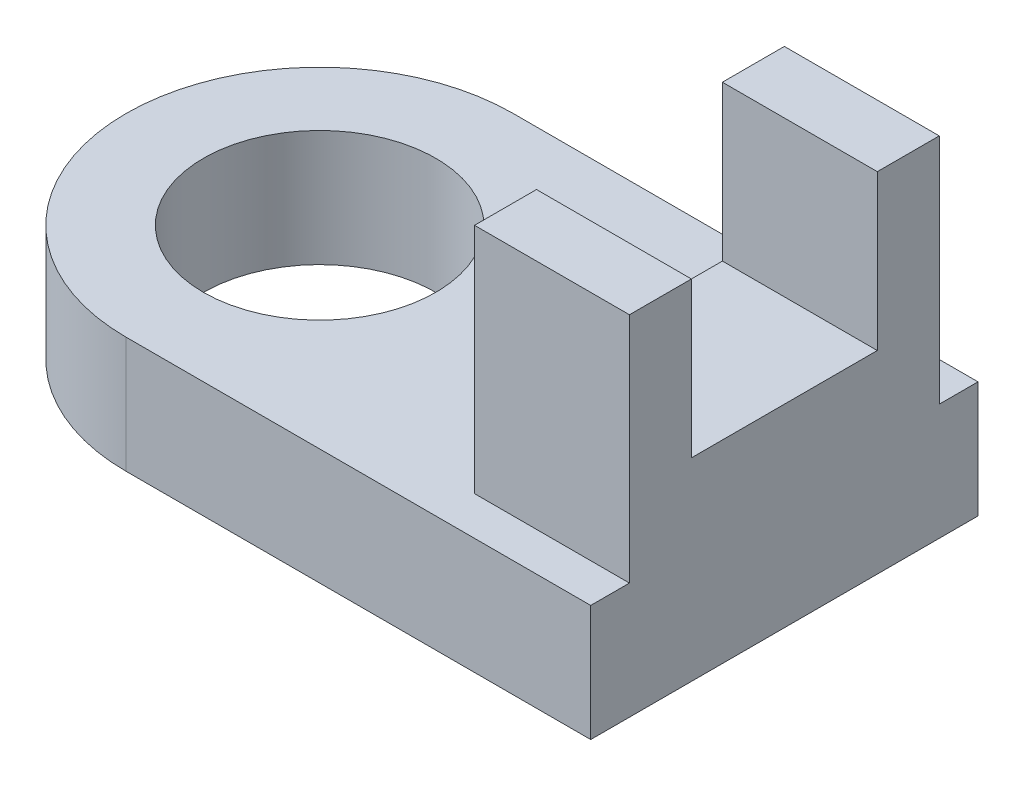
ISO-10303-21;
HEADER;
FILE_DESCRIPTION(('STEP AP214'),'2;1');
FILE_NAME('part.step','',(''),(''),'','','');
FILE_SCHEMA(('AUTOMOTIVE_DESIGN { 1 0 10303 214 1 1 1 1 }'));
ENDSEC;
DATA;
#1=APPLICATION_CONTEXT('core data for automotive mechanical design processes');
#2=APPLICATION_PROTOCOL_DEFINITION('international standard','automotive_design',2000,#1);
#3=PRODUCT_CONTEXT('',#1,'mechanical');
#4=PRODUCT('Part','Part','',(#3));
#5=PRODUCT_RELATED_PRODUCT_CATEGORY('part','',(#4));
#6=PRODUCT_DEFINITION_FORMATION('','',#4);
#7=PRODUCT_DEFINITION_CONTEXT('part definition',#1,'design');
#8=PRODUCT_DEFINITION('design','',#6,#7);
#9=PRODUCT_DEFINITION_SHAPE('','',#8);
#10=(LENGTH_UNIT() NAMED_UNIT(*) SI_UNIT(.MILLI.,.METRE.));
#11=(NAMED_UNIT(*) PLANE_ANGLE_UNIT() SI_UNIT($,.RADIAN.));
#12=(NAMED_UNIT(*) SI_UNIT($,.STERADIAN.) SOLID_ANGLE_UNIT());
#13=UNCERTAINTY_MEASURE_WITH_UNIT(LENGTH_MEASURE(1.E-05),#10,'distance_accuracy_value','');
#14=(GEOMETRIC_REPRESENTATION_CONTEXT(3) GLOBAL_UNCERTAINTY_ASSIGNED_CONTEXT((#13)) GLOBAL_UNIT_ASSIGNED_CONTEXT((#10,
#11,#12)) REPRESENTATION_CONTEXT('',''));
#15=CARTESIAN_POINT('',(0.,0.,0.));
#16=DIRECTION('',(0.,0.,1.));
#17=DIRECTION('',(1.,0.,0.));
#18=AXIS2_PLACEMENT_3D('',#15,#16,#17);
#19=CARTESIAN_POINT('',(-30.,7.5,25.));
#20=DIRECTION('',(0.,-1.,0.));
#21=DIRECTION('',(0.,0.,-1.));
#22=AXIS2_PLACEMENT_3D('',#19,#20,#21);
#23=PLANE('',#22);
#24=CARTESIAN_POINT('',(-30.,7.5,0.));
#25=DIRECTION('',(0.,1.,0.));
#26=DIRECTION('',(0.,0.,1.));
#27=AXIS2_PLACEMENT_3D('',#24,#25,#26);
#28=CIRCLE('',#27,15.);
#29=CARTESIAN_POINT('',(-30.,7.5,15.));
#30=VERTEX_POINT('',#29);
#31=EDGE_CURVE('E160',#30,#30,#28,.T.);
#32=ORIENTED_EDGE('',*,*,#31,.F.);
#33=EDGE_LOOP('',(#32));
#34=FACE_BOUND('',#33,.T.);
#35=DIRECTION('',(1.,0.,0.));
#36=VECTOR('',#35,1.);
#37=CARTESIAN_POINT('',(10.,7.49999999999999,20.));
#38=LINE('',#37,#36);
#39=CARTESIAN_POINT('',(10.,7.49999999999999,20.));
#40=VERTEX_POINT('',#39);
#41=CARTESIAN_POINT('',(30.,7.5,20.));
#42=VERTEX_POINT('',#41);
#43=EDGE_CURVE('E207',#40,#42,#38,.T.);
#44=ORIENTED_EDGE('',*,*,#43,.F.);
#45=DIRECTION('',(0.,0.,-1.));
#46=VECTOR('',#45,1.);
#47=CARTESIAN_POINT('',(10.,7.5,-20.));
#48=LINE('',#47,#46);
#49=CARTESIAN_POINT('',(10.,7.5,-20.));
#50=VERTEX_POINT('',#49);
#51=EDGE_CURVE('E164',#40,#50,#48,.T.);
#52=ORIENTED_EDGE('',*,*,#51,.T.);
#53=DIRECTION('',(1.,0.,0.));
#54=VECTOR('',#53,1.);
#55=CARTESIAN_POINT('',(10.,7.5,-20.));
#56=LINE('',#55,#54);
#57=CARTESIAN_POINT('',(30.,7.5,-20.));
#58=VERTEX_POINT('',#57);
#59=EDGE_CURVE('E187',#50,#58,#56,.T.);
#60=ORIENTED_EDGE('',*,*,#59,.T.);
#61=DIRECTION('',(0.,0.,-1.));
#62=VECTOR('',#61,1.);
#63=CARTESIAN_POINT('',(30.,7.5,25.));
#64=LINE('',#63,#62);
#65=CARTESIAN_POINT('',(30.,7.5,-25.));
#66=VERTEX_POINT('',#65);
#67=EDGE_CURVE('E47',#58,#66,#64,.T.);
#68=ORIENTED_EDGE('',*,*,#67,.T.);
#69=DIRECTION('',(-1.,0.,0.));
#70=VECTOR('',#69,1.);
#71=CARTESIAN_POINT('',(-30.,7.5,-25.));
#72=LINE('',#71,#70);
#73=CARTESIAN_POINT('',(-30.,7.5,-25.));
#74=VERTEX_POINT('',#73);
#75=EDGE_CURVE('E153',#66,#74,#72,.T.);
#76=ORIENTED_EDGE('',*,*,#75,.T.);
#77=CARTESIAN_POINT('',(-30.,7.5,0.));
#78=DIRECTION('',(0.,1.,0.));
#79=DIRECTION('',(0.,0.,1.));
#80=AXIS2_PLACEMENT_3D('',#77,#78,#79);
#81=CIRCLE('',#80,25.);
#82=CARTESIAN_POINT('',(-30.,7.5,25.));
#83=VERTEX_POINT('',#82);
#84=EDGE_CURVE('E155',#74,#83,#81,.T.);
#85=ORIENTED_EDGE('',*,*,#84,.T.);
#86=DIRECTION('',(-1.,0.,0.));
#87=VECTOR('',#86,1.);
#88=CARTESIAN_POINT('',(-30.,7.5,25.));
#89=LINE('',#88,#87);
#90=CARTESIAN_POINT('',(30.,7.5,25.));
#91=VERTEX_POINT('',#90);
#92=EDGE_CURVE('E90',#91,#83,#89,.T.);
#93=ORIENTED_EDGE('',*,*,#92,.F.);
#94=EDGE_CURVE('E11',#91,#42,#64,.T.);
#95=ORIENTED_EDGE('',*,*,#94,.T.);
#96=EDGE_LOOP('',(#44,#52,#60,#68,#76,#85,#93,#95));
#97=FACE_BOUND('',#96,.T.);
#98=ADVANCED_FACE('F41',(#34,#97),#23,.F.);
#99=CARTESIAN_POINT('',(30.,7.5,25.));
#100=DIRECTION('',(-1.,0.,0.));
#101=DIRECTION('',(0.,-1.,0.));
#102=AXIS2_PLACEMENT_3D('',#99,#100,#101);
#103=PLANE('',#102);
#104=DIRECTION('',(0.,1.,0.));
#105=VECTOR('',#104,1.);
#106=CARTESIAN_POINT('',(30.,7.5,-25.));
#107=LINE('',#106,#105);
#108=CARTESIAN_POINT('',(30.,-7.5,-25.));
#109=VERTEX_POINT('',#108);
#110=EDGE_CURVE('E148',#109,#66,#107,.T.);
#111=ORIENTED_EDGE('',*,*,#110,.T.);
#112=ORIENTED_EDGE('',*,*,#67,.F.);
#113=DIRECTION('',(0.,1.,0.));
#114=VECTOR('',#113,1.);
#115=CARTESIAN_POINT('',(30.,37.5,-20.));
#116=LINE('',#115,#114);
#117=CARTESIAN_POINT('',(30.,37.5,-20.));
#118=VERTEX_POINT('',#117);
#119=EDGE_CURVE('E57',#58,#118,#116,.T.);
#120=ORIENTED_EDGE('',*,*,#119,.T.);
#121=DIRECTION('',(0.,0.,1.));
#122=VECTOR('',#121,1.);
#123=CARTESIAN_POINT('',(30.,37.5,-12.));
#124=LINE('',#123,#122);
#125=CARTESIAN_POINT('',(30.,37.5,-12.));
#126=VERTEX_POINT('',#125);
#127=EDGE_CURVE('E195',#118,#126,#124,.T.);
#128=ORIENTED_EDGE('',*,*,#127,.T.);
#129=DIRECTION('',(0.,-1.,0.));
#130=VECTOR('',#129,1.);
#131=CARTESIAN_POINT('',(30.,17.5,-12.));
#132=LINE('',#131,#130);
#133=CARTESIAN_POINT('',(30.,17.5,-12.));
#134=VERTEX_POINT('',#133);
#135=EDGE_CURVE('E192',#126,#134,#132,.T.);
#136=ORIENTED_EDGE('',*,*,#135,.T.);
#137=DIRECTION('',(0.,0.,1.));
#138=VECTOR('',#137,1.);
#139=CARTESIAN_POINT('',(30.,17.5,12.));
#140=LINE('',#139,#138);
#141=CARTESIAN_POINT('',(30.,17.5,12.));
#142=VERTEX_POINT('',#141);
#143=EDGE_CURVE('E196',#134,#142,#140,.T.);
#144=ORIENTED_EDGE('',*,*,#143,.T.);
#145=DIRECTION('',(0.,1.,0.));
#146=VECTOR('',#145,1.);
#147=CARTESIAN_POINT('',(30.,37.5,12.));
#148=LINE('',#147,#146);
#149=CARTESIAN_POINT('',(30.,37.5,12.));
#150=VERTEX_POINT('',#149);
#151=EDGE_CURVE('E203',#142,#150,#148,.T.);
#152=ORIENTED_EDGE('',*,*,#151,.T.);
#153=DIRECTION('',(0.,0.,1.));
#154=VECTOR('',#153,1.);
#155=CARTESIAN_POINT('',(30.,37.5,20.));
#156=LINE('',#155,#154);
#157=CARTESIAN_POINT('',(30.,37.5,20.));
#158=VERTEX_POINT('',#157);
#159=EDGE_CURVE('E204',#150,#158,#156,.T.);
#160=ORIENTED_EDGE('',*,*,#159,.T.);
#161=DIRECTION('',(0.,-1.,0.));
#162=VECTOR('',#161,1.);
#163=CARTESIAN_POINT('',(30.,7.5,20.));
#164=LINE('',#163,#162);
#165=EDGE_CURVE('E166',#158,#42,#164,.T.);
#166=ORIENTED_EDGE('',*,*,#165,.T.);
#167=ORIENTED_EDGE('',*,*,#94,.F.);
#168=DIRECTION('',(0.,1.,0.));
#169=VECTOR('',#168,1.);
#170=CARTESIAN_POINT('',(30.,7.5,25.));
#171=LINE('',#170,#169);
#172=CARTESIAN_POINT('',(30.,-7.5,25.));
#173=VERTEX_POINT('',#172);
#174=EDGE_CURVE('E150',#173,#91,#171,.T.);
#175=ORIENTED_EDGE('',*,*,#174,.F.);
#176=DIRECTION('',(0.,0.,-1.));
#177=VECTOR('',#176,1.);
#178=CARTESIAN_POINT('',(30.,-7.5,25.));
#179=LINE('',#178,#177);
#180=EDGE_CURVE('E228',#173,#109,#179,.T.);
#181=ORIENTED_EDGE('',*,*,#180,.T.);
#182=EDGE_LOOP('',(#111,#112,#120,#128,#136,#144,#152,#160,#166,#167,#175,#181));
#183=FACE_BOUND('',#182,.T.);
#184=ADVANCED_FACE('F43',(#183),#103,.F.);
#185=CARTESIAN_POINT('',(-30.,-7.5,25.));
#186=DIRECTION('',(0.,1.,0.));
#187=DIRECTION('',(0.,0.,1.));
#188=AXIS2_PLACEMENT_3D('',#185,#186,#187);
#189=PLANE('',#188);
#190=CARTESIAN_POINT('',(-30.,-7.5,0.));
#191=DIRECTION('',(0.,1.,0.));
#192=DIRECTION('',(0.,0.,1.));
#193=AXIS2_PLACEMENT_3D('',#190,#191,#192);
#194=CIRCLE('',#193,15.);
#195=CARTESIAN_POINT('',(-30.,-7.5,15.));
#196=VERTEX_POINT('',#195);
#197=EDGE_CURVE('E156',#196,#196,#194,.T.);
#198=ORIENTED_EDGE('',*,*,#197,.T.);
#199=EDGE_LOOP('',(#198));
#200=FACE_BOUND('',#199,.T.);
#201=DIRECTION('',(1.,0.,0.));
#202=VECTOR('',#201,1.);
#203=CARTESIAN_POINT('',(-30.,-7.5,-25.));
#204=LINE('',#203,#202);
#205=CARTESIAN_POINT('',(-30.,-7.5,-25.));
#206=VERTEX_POINT('',#205);
#207=EDGE_CURVE('E81',#206,#109,#204,.T.);
#208=ORIENTED_EDGE('',*,*,#207,.T.);
#209=ORIENTED_EDGE('',*,*,#180,.F.);
#210=DIRECTION('',(1.,0.,0.));
#211=VECTOR('',#210,1.);
#212=CARTESIAN_POINT('',(-30.,-7.5,25.));
#213=LINE('',#212,#211);
#214=CARTESIAN_POINT('',(-30.,-7.5,25.));
#215=VERTEX_POINT('',#214);
#216=EDGE_CURVE('E62',#215,#173,#213,.T.);
#217=ORIENTED_EDGE('',*,*,#216,.F.);
#218=CARTESIAN_POINT('',(-30.,-7.5,0.));
#219=DIRECTION('',(0.,1.,0.));
#220=DIRECTION('',(0.,0.,1.));
#221=AXIS2_PLACEMENT_3D('',#218,#219,#220);
#222=CIRCLE('',#221,25.);
#223=EDGE_CURVE('E151',#206,#215,#222,.T.);
#224=ORIENTED_EDGE('',*,*,#223,.F.);
#225=EDGE_LOOP('',(#208,#209,#217,#224));
#226=FACE_BOUND('',#225,.T.);
#227=ADVANCED_FACE('F154',(#200,#226),#189,.F.);
#228=CARTESIAN_POINT('',(0.,0.,25.));
#229=DIRECTION('',(0.,0.,1.));
#230=DIRECTION('',(1.,0.,0.));
#231=AXIS2_PLACEMENT_3D('',#228,#229,#230);
#232=PLANE('',#231);
#233=ORIENTED_EDGE('',*,*,#174,.T.);
#234=ORIENTED_EDGE('',*,*,#92,.T.);
#235=DIRECTION('',(0.,-1.,0.));
#236=VECTOR('',#235,1.);
#237=CARTESIAN_POINT('',(-30.,7.5,25.));
#238=LINE('',#237,#236);
#239=EDGE_CURVE('E229',#83,#215,#238,.T.);
#240=ORIENTED_EDGE('',*,*,#239,.T.);
#241=ORIENTED_EDGE('',*,*,#216,.T.);
#242=EDGE_LOOP('',(#233,#234,#240,#241));
#243=FACE_BOUND('',#242,.T.);
#244=ADVANCED_FACE('F238',(#243),#232,.T.);
#245=CARTESIAN_POINT('',(0.,0.,-25.));
#246=DIRECTION('',(0.,0.,1.));
#247=DIRECTION('',(1.,0.,0.));
#248=AXIS2_PLACEMENT_3D('',#245,#246,#247);
#249=PLANE('',#248);
#250=ORIENTED_EDGE('',*,*,#110,.F.);
#251=ORIENTED_EDGE('',*,*,#207,.F.);
#252=DIRECTION('',(0.,-1.,0.));
#253=VECTOR('',#252,1.);
#254=CARTESIAN_POINT('',(-30.,7.5,-25.));
#255=LINE('',#254,#253);
#256=EDGE_CURVE('E141',#74,#206,#255,.T.);
#257=ORIENTED_EDGE('',*,*,#256,.F.);
#258=ORIENTED_EDGE('',*,*,#75,.F.);
#259=EDGE_LOOP('',(#250,#251,#257,#258));
#260=FACE_BOUND('',#259,.T.);
#261=ADVANCED_FACE('F143',(#260),#249,.F.);
#262=CARTESIAN_POINT('',(10.,7.49999999999999,20.));
#263=DIRECTION('',(0.,0.,1.));
#264=DIRECTION('',(1.,0.,0.));
#265=AXIS2_PLACEMENT_3D('',#262,#263,#264);
#266=PLANE('',#265);
#267=ORIENTED_EDGE('',*,*,#165,.F.);
#268=DIRECTION('',(1.,0.,0.));
#269=VECTOR('',#268,1.);
#270=CARTESIAN_POINT('',(9.99999999999999,37.5,20.));
#271=LINE('',#270,#269);
#272=CARTESIAN_POINT('',(9.99999999999999,37.5,20.));
#273=VERTEX_POINT('',#272);
#274=EDGE_CURVE('E211',#273,#158,#271,.T.);
#275=ORIENTED_EDGE('',*,*,#274,.F.);
#276=DIRECTION('',(0.,-1.,0.));
#277=VECTOR('',#276,1.);
#278=CARTESIAN_POINT('',(10.,7.49999999999999,20.));
#279=LINE('',#278,#277);
#280=EDGE_CURVE('E186',#273,#40,#279,.T.);
#281=ORIENTED_EDGE('',*,*,#280,.T.);
#282=ORIENTED_EDGE('',*,*,#43,.T.);
#283=EDGE_LOOP('',(#267,#275,#281,#282));
#284=FACE_BOUND('',#283,.T.);
#285=ADVANCED_FACE('F252',(#284),#266,.T.);
#286=CARTESIAN_POINT('',(9.99999999999999,37.5,20.));
#287=DIRECTION('',(0.,1.,0.));
#288=DIRECTION('',(-1.,0.,0.));
#289=AXIS2_PLACEMENT_3D('',#286,#287,#288);
#290=PLANE('',#289);
#291=ORIENTED_EDGE('',*,*,#159,.F.);
#292=DIRECTION('',(1.,0.,0.));
#293=VECTOR('',#292,1.);
#294=CARTESIAN_POINT('',(9.99999999999999,37.5,12.));
#295=LINE('',#294,#293);
#296=CARTESIAN_POINT('',(9.99999999999999,37.5,12.));
#297=VERTEX_POINT('',#296);
#298=EDGE_CURVE('E213',#297,#150,#295,.T.);
#299=ORIENTED_EDGE('',*,*,#298,.F.);
#300=DIRECTION('',(0.,0.,1.));
#301=VECTOR('',#300,1.);
#302=CARTESIAN_POINT('',(9.99999999999999,37.5,20.));
#303=LINE('',#302,#301);
#304=EDGE_CURVE('E184',#297,#273,#303,.T.);
#305=ORIENTED_EDGE('',*,*,#304,.T.);
#306=ORIENTED_EDGE('',*,*,#274,.T.);
#307=EDGE_LOOP('',(#291,#299,#305,#306));
#308=FACE_BOUND('',#307,.T.);
#309=ADVANCED_FACE('F273',(#308),#290,.T.);
#310=CARTESIAN_POINT('',(9.99999999999999,37.5,12.));
#311=DIRECTION('',(0.,0.,-1.));
#312=DIRECTION('',(0.,1.,0.));
#313=AXIS2_PLACEMENT_3D('',#310,#311,#312);
#314=PLANE('',#313);
#315=ORIENTED_EDGE('',*,*,#151,.F.);
#316=DIRECTION('',(1.,0.,0.));
#317=VECTOR('',#316,1.);
#318=CARTESIAN_POINT('',(10.,17.5,12.));
#319=LINE('',#318,#317);
#320=CARTESIAN_POINT('',(10.,17.5,12.));
#321=VERTEX_POINT('',#320);
#322=EDGE_CURVE('E214',#321,#142,#319,.T.);
#323=ORIENTED_EDGE('',*,*,#322,.F.);
#324=DIRECTION('',(0.,1.,0.));
#325=VECTOR('',#324,1.);
#326=CARTESIAN_POINT('',(9.99999999999999,37.5,12.));
#327=LINE('',#326,#325);
#328=EDGE_CURVE('E182',#321,#297,#327,.T.);
#329=ORIENTED_EDGE('',*,*,#328,.T.);
#330=ORIENTED_EDGE('',*,*,#298,.T.);
#331=EDGE_LOOP('',(#315,#323,#329,#330));
#332=FACE_BOUND('',#331,.T.);
#333=ADVANCED_FACE('F269',(#332),#314,.T.);
#334=CARTESIAN_POINT('',(10.,17.5,12.));
#335=DIRECTION('',(0.,1.,0.));
#336=DIRECTION('',(-1.,0.,0.));
#337=AXIS2_PLACEMENT_3D('',#334,#335,#336);
#338=PLANE('',#337);
#339=ORIENTED_EDGE('',*,*,#143,.F.);
#340=DIRECTION('',(1.,0.,0.));
#341=VECTOR('',#340,1.);
#342=CARTESIAN_POINT('',(10.,17.5,-12.));
#343=LINE('',#342,#341);
#344=CARTESIAN_POINT('',(10.,17.5,-12.));
#345=VERTEX_POINT('',#344);
#346=EDGE_CURVE('E220',#345,#134,#343,.T.);
#347=ORIENTED_EDGE('',*,*,#346,.F.);
#348=DIRECTION('',(0.,0.,1.));
#349=VECTOR('',#348,1.);
#350=CARTESIAN_POINT('',(10.,17.5,12.));
#351=LINE('',#350,#349);
#352=EDGE_CURVE('E176',#345,#321,#351,.T.);
#353=ORIENTED_EDGE('',*,*,#352,.T.);
#354=ORIENTED_EDGE('',*,*,#322,.T.);
#355=EDGE_LOOP('',(#339,#347,#353,#354));
#356=FACE_BOUND('',#355,.T.);
#357=ADVANCED_FACE('F266',(#356),#338,.T.);
#358=CARTESIAN_POINT('',(10.,17.5,-12.));
#359=DIRECTION('',(0.,0.,1.));
#360=DIRECTION('',(1.,0.,0.));
#361=AXIS2_PLACEMENT_3D('',#358,#359,#360);
#362=PLANE('',#361);
#363=ORIENTED_EDGE('',*,*,#135,.F.);
#364=DIRECTION('',(1.,0.,0.));
#365=VECTOR('',#364,1.);
#366=CARTESIAN_POINT('',(9.99999999999999,37.5,-12.));
#367=LINE('',#366,#365);
#368=CARTESIAN_POINT('',(9.99999999999999,37.5,-12.));
#369=VERTEX_POINT('',#368);
#370=EDGE_CURVE('E218',#369,#126,#367,.T.);
#371=ORIENTED_EDGE('',*,*,#370,.F.);
#372=DIRECTION('',(0.,-1.,0.));
#373=VECTOR('',#372,1.);
#374=CARTESIAN_POINT('',(10.,17.5,-12.));
#375=LINE('',#374,#373);
#376=EDGE_CURVE('E172',#369,#345,#375,.T.);
#377=ORIENTED_EDGE('',*,*,#376,.T.);
#378=ORIENTED_EDGE('',*,*,#346,.T.);
#379=EDGE_LOOP('',(#363,#371,#377,#378));
#380=FACE_BOUND('',#379,.T.);
#381=ADVANCED_FACE('F265',(#380),#362,.T.);
#382=CARTESIAN_POINT('',(9.99999999999999,37.5,-12.));
#383=DIRECTION('',(0.,1.,0.));
#384=DIRECTION('',(-1.,0.,0.));
#385=AXIS2_PLACEMENT_3D('',#382,#383,#384);
#386=PLANE('',#385);
#387=ORIENTED_EDGE('',*,*,#127,.F.);
#388=DIRECTION('',(1.,0.,0.));
#389=VECTOR('',#388,1.);
#390=CARTESIAN_POINT('',(9.99999999999999,37.5,-20.));
#391=LINE('',#390,#389);
#392=CARTESIAN_POINT('',(9.99999999999999,37.5,-20.));
#393=VERTEX_POINT('',#392);
#394=EDGE_CURVE('E222',#393,#118,#391,.T.);
#395=ORIENTED_EDGE('',*,*,#394,.F.);
#396=DIRECTION('',(0.,0.,1.));
#397=VECTOR('',#396,1.);
#398=CARTESIAN_POINT('',(9.99999999999999,37.5,-12.));
#399=LINE('',#398,#397);
#400=EDGE_CURVE('E171',#393,#369,#399,.T.);
#401=ORIENTED_EDGE('',*,*,#400,.T.);
#402=ORIENTED_EDGE('',*,*,#370,.T.);
#403=EDGE_LOOP('',(#387,#395,#401,#402));
#404=FACE_BOUND('',#403,.T.);
#405=ADVANCED_FACE('F259',(#404),#386,.T.);
#406=CARTESIAN_POINT('',(9.99999999999999,37.5,-20.));
#407=DIRECTION('',(0.,0.,-1.));
#408=DIRECTION('',(-1.,0.,0.));
#409=AXIS2_PLACEMENT_3D('',#406,#407,#408);
#410=PLANE('',#409);
#411=ORIENTED_EDGE('',*,*,#119,.F.);
#412=ORIENTED_EDGE('',*,*,#59,.F.);
#413=DIRECTION('',(0.,1.,0.));
#414=VECTOR('',#413,1.);
#415=CARTESIAN_POINT('',(9.99999999999999,37.5,-20.));
#416=LINE('',#415,#414);
#417=EDGE_CURVE('E169',#50,#393,#416,.T.);
#418=ORIENTED_EDGE('',*,*,#417,.T.);
#419=ORIENTED_EDGE('',*,*,#394,.T.);
#420=EDGE_LOOP('',(#411,#412,#418,#419));
#421=FACE_BOUND('',#420,.T.);
#422=ADVANCED_FACE('F254',(#421),#410,.T.);
#423=CARTESIAN_POINT('',(10.,0.,0.));
#424=DIRECTION('',(-1.,0.,0.));
#425=DIRECTION('',(0.,-1.,0.));
#426=AXIS2_PLACEMENT_3D('',#423,#424,#425);
#427=PLANE('',#426);
#428=ORIENTED_EDGE('',*,*,#51,.F.);
#429=ORIENTED_EDGE('',*,*,#280,.F.);
#430=ORIENTED_EDGE('',*,*,#304,.F.);
#431=ORIENTED_EDGE('',*,*,#328,.F.);
#432=ORIENTED_EDGE('',*,*,#352,.F.);
#433=ORIENTED_EDGE('',*,*,#376,.F.);
#434=ORIENTED_EDGE('',*,*,#400,.F.);
#435=ORIENTED_EDGE('',*,*,#417,.F.);
#436=EDGE_LOOP('',(#428,#429,#430,#431,#432,#433,#434,#435));
#437=FACE_BOUND('',#436,.T.);
#438=ADVANCED_FACE('F256',(#437),#427,.T.);
#439=CARTESIAN_POINT('',(-30.,-7.5,0.));
#440=DIRECTION('',(0.,1.,0.));
#441=DIRECTION('',(0.,0.,1.));
#442=AXIS2_PLACEMENT_3D('',#439,#440,#441);
#443=CYLINDRICAL_SURFACE('',#442,15.);
#444=ORIENTED_EDGE('',*,*,#31,.T.);
#445=EDGE_LOOP('',(#444));
#446=FACE_BOUND('',#445,.T.);
#447=ORIENTED_EDGE('',*,*,#197,.F.);
#448=EDGE_LOOP('',(#447));
#449=FACE_BOUND('',#448,.T.);
#450=ADVANCED_FACE('F285',(#446,#449),#443,.F.);
#451=CARTESIAN_POINT('',(-30.,-7.5,0.));
#452=DIRECTION('',(0.,1.,0.));
#453=DIRECTION('',(0.,0.,1.));
#454=AXIS2_PLACEMENT_3D('',#451,#452,#453);
#455=CYLINDRICAL_SURFACE('',#454,25.);
#456=ORIENTED_EDGE('',*,*,#84,.F.);
#457=ORIENTED_EDGE('',*,*,#256,.T.);
#458=ORIENTED_EDGE('',*,*,#223,.T.);
#459=ORIENTED_EDGE('',*,*,#239,.F.);
#460=EDGE_LOOP('',(#456,#457,#458,#459));
#461=FACE_BOUND('',#460,.T.);
#462=ADVANCED_FACE('F147',(#461),#455,.T.);
#463=CLOSED_SHELL('',(#98,#184,#227,#244,#261,#285,#309,#333,#357,#381,#405,#422,#438,#450,#462));
#464=MANIFOLD_SOLID_BREP('B2',#463);
#465=ADVANCED_BREP_SHAPE_REPRESENTATION('',(#18,#464),#14);
#466=SHAPE_DEFINITION_REPRESENTATION(#9,#465);
ENDSEC;
END-ISO-10303-21;
